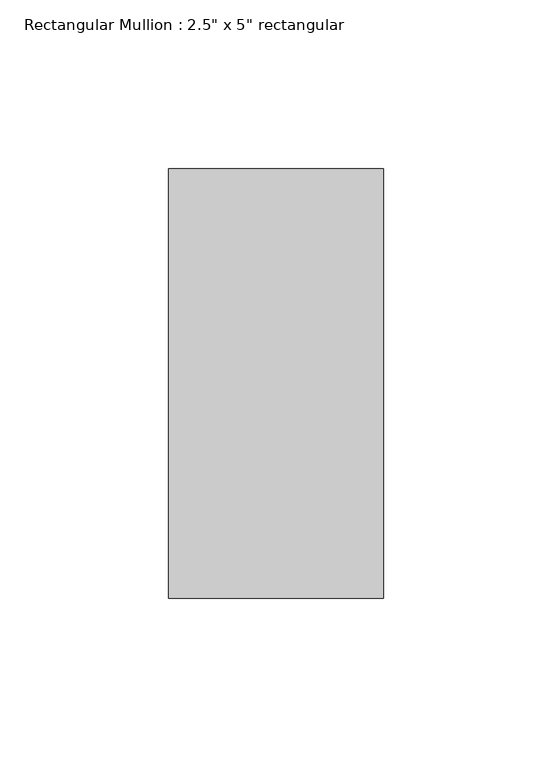
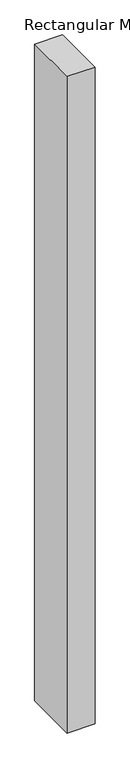
"""IFC4 building model written with IfcOpenShell, lengths in millimetres: member geometry."""

from ifc_helpers import new_model, si_unit, frame, origin, place, context, project, spatial, polyline, outline, extrude, source, transform, mapped, element, save


def member_7ceeb836(model_context):
    return source(origin(), model_context, "Body", "SweptSolid", [
        extrude(outline(polyline([(31.75, 63.5), (31.75, -63.5), (-31.75, -63.5), (-31.75, 63.5), (31.75, 63.5)])), frame((0.0, 0.0, -1573.6725209), z_axis=(0.0, 0.0, 1.0), x_axis=(1.0, 0.0, 0.0)), (0.0, 0.0, 1.0), 1573.6725209),
    ])


if __name__ == "__main__":
    model = new_model("IFC4")
    model_context = context("Model", 3, world=origin())
    ifc_project = project(units=[si_unit("LENGTHUNIT", "METRE", prefix="MILLI")], contexts=[model_context])
    site = spatial("IfcSite", under=ifc_project)
    building = spatial("IfcBuilding", under=site)
    placement = place(None, origin())
    member_shape = member_7ceeb836(model_context)
    element("IfcMember", 1, ObjectType="Rectangular Mullion : 2.5\" x 5\" rectangular", at=placement, inside=building, context=model_context, shape_type="MappedRepresentation", body=[
        mapped(member_shape, transform((0.0, 0.0, 0.0), x_axis=(1.0, 0.0, 0.0), y_axis=(0.0, 1.0, 0.0), z_axis=(0.0, 0.0, 1.0))),
    ])
    save(model, "model.ifc")

# Revit data of these elements
# Type "Rectangular Mullion : 2.5\" x 5\" rectangular"
#   built-in parameter 1007304 = 0.416667 (stored number, unit not read)
#   built-in parameter 1007301 = 0.104167 (stored number, unit not read)
#   built-in parameter 1007300 = 0.104167 (stored number, unit not read)
# Element 1 (IfcMember, "Rectangular Mullion : 2.5\" x 5\" rectangular")
#   Materials on its faces: "Aluminum"
# Materials
#   "Aluminum": class "Metal", colour RGB 247 247 247, transparency 0, Description = "Aluminum 6061", Cost = 0
